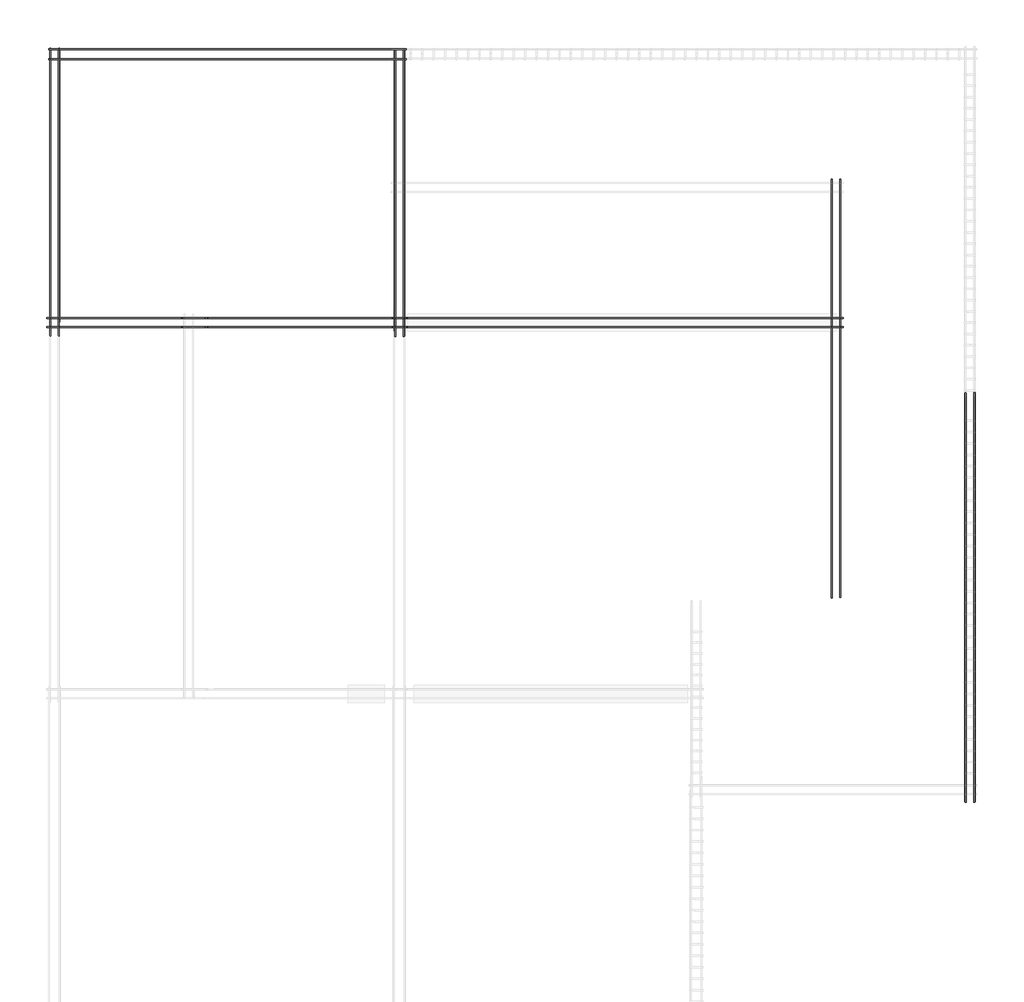
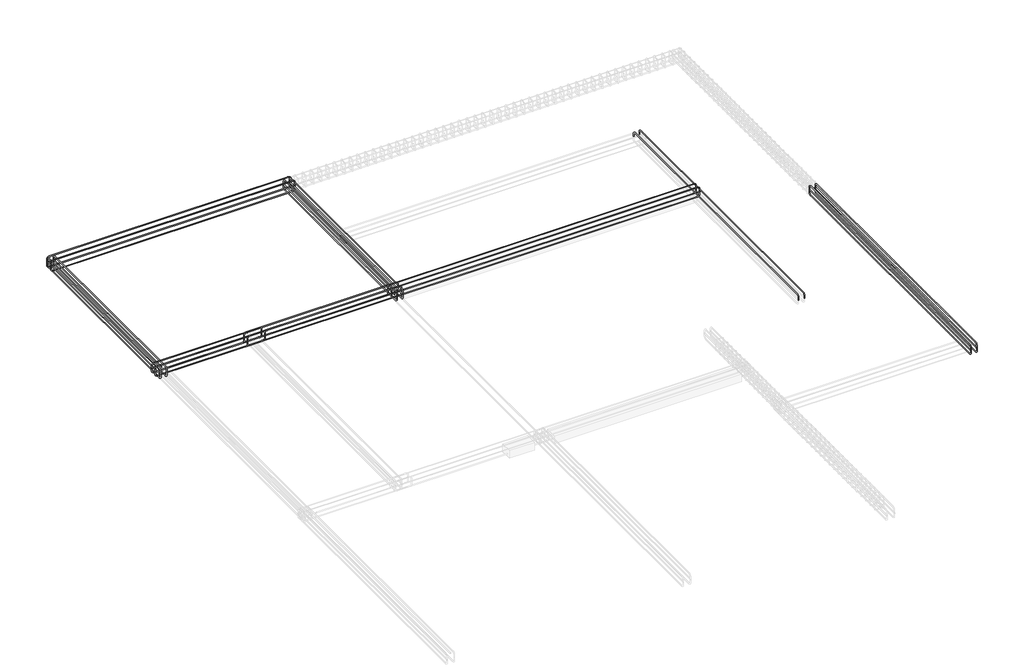
# One storey, part 4 of 5: 44 reinforcing bars.
"""IFC4 building model written with IfcOpenShell, lengths in millimetres."""

from ifc_helpers import new_model, si_unit, point, frame, origin, place, context, project, spatial, polyline, circle_curve, trimmed, segment, composite_curve, element, save
from ifc_brep_helpers import swept_disk

model = new_model("IFC4")

# Units and contexts
model_context = context("Model", 3, world=origin())
ifc_project = project(units=[si_unit("LENGTHUNIT", "METRE", prefix="MILLI")], contexts=[model_context])

# Site, building, storey
site = spatial("IfcSite", under=ifc_project)
building = spatial("IfcBuilding", under=site)
storey = spatial("IfcBuildingStorey", under=building, Elevation=0.0)

# Reinforcing bars
placement = place(None, origin())
element("IfcReinforcingBar", 1, at=placement, inside=storey, context=model_context, shape_type="SolidModel", body=[
    swept_disk(composite_curve([segment(polyline([(-10115.1918223, 13372.4913561, 314.2193272), (-10115.1918223, 13372.4913561, 365.0193272)]), True, "CONTINUOUS"), segment(trimmed(circle_curve(frame((-10159.6418223, 13372.4913561, 365.0193272), z_axis=(0.0, -1.0, 0.0), x_axis=(44.45000000000073, 0.0, 0.0)), 44.45), [point((-10115.1918223, 13372.4913561, 365.0193272))], [point((-10159.6418223, 13372.4913561, 409.4693272))], True, "CARTESIAN"), True, "CONTINUOUS"), segment(polyline([(-10159.6418223, 13372.4913561, 409.4693272), (-14737.9918223, 13372.4913561, 409.4693272)]), True, "CONTINUOUS"), segment(trimmed(circle_curve(frame((-14737.9918223, 13372.4913561, 365.0193272), z_axis=(0.0, -1.0, 0.0), x_axis=(0.0, 0.0, 44.44999999999999)), 44.45), [point((-14737.9918223, 13372.4913561, 409.4693272))], [point((-14782.4418223, 13372.4913561, 365.0193272))], True, "CARTESIAN"), True, "CONTINUOUS"), segment(polyline([(-14782.4418223, 13372.4913561, 365.0193272), (-14782.4418223, 13372.4913561, 314.2193272)]), True, "CONTINUOUS")], self_intersect=False), 6.35),
])
element("IfcReinforcingBar", 2, at=placement, inside=storey, context=model_context, shape_type="SolidModel", body=[
    swept_disk(composite_curve([segment(polyline([(-10115.1918223, 13244.7305243, 314.2193272), (-10115.1918223, 13244.7305243, 365.0193272)]), True, "CONTINUOUS"), segment(trimmed(circle_curve(frame((-10159.6418223, 13244.7305243, 365.0193272), z_axis=(0.0, -1.0, 0.0), x_axis=(44.45000000000073, 0.0, 0.0)), 44.45), [point((-10115.1918223, 13244.7305243, 365.0193272))], [point((-10159.6418223, 13244.7305243, 409.4693272))], True, "CARTESIAN"), True, "CONTINUOUS"), segment(polyline([(-10159.6418223, 13244.7305243, 409.4693272), (-14737.9918223, 13244.7305243, 409.4693272)]), True, "CONTINUOUS"), segment(trimmed(circle_curve(frame((-14737.9918223, 13244.7305243, 365.0193272), z_axis=(0.0, -1.0, 0.0), x_axis=(0.0, 0.0, 44.44999999999999)), 44.45), [point((-14737.9918223, 13244.7305243, 409.4693272))], [point((-14782.4418223, 13244.7305243, 365.0193272))], True, "CARTESIAN"), True, "CONTINUOUS"), segment(polyline([(-14782.4418223, 13244.7305243, 365.0193272), (-14782.4418223, 13244.7305243, 314.2193272)]), True, "CONTINUOUS")], self_intersect=False), 6.35),
])
element("IfcReinforcingBar", 3, at=placement, inside=storey, context=model_context, shape_type="SolidModel", body=[
    swept_disk(composite_curve([segment(polyline([(-10115.1918223, 13372.4913561, 295.3806728), (-10115.1918223, 13372.4913561, 244.5806728)]), True, "CONTINUOUS"), segment(trimmed(circle_curve(frame((-10159.6418223, 13372.4913561, 244.5806728), z_axis=(0.0, 1.0, 0.0), x_axis=(44.45000000000073, 0.0, 0.0)), 44.45), [point((-10115.1918223, 13372.4913561, 244.5806728))], [point((-10159.6418223, 13372.4913561, 200.1306728))], True, "CARTESIAN"), True, "CONTINUOUS"), segment(polyline([(-10159.6418223, 13372.4913561, 200.1306728), (-14737.9918223, 13372.4913561, 200.1306728)]), True, "CONTINUOUS"), segment(trimmed(circle_curve(frame((-14737.9918223, 13372.4913561, 244.5806728), z_axis=(0.0, 1.0, 0.0), x_axis=(0.0, 0.0, -44.44999999999999)), 44.45), [point((-14737.9918223, 13372.4913561, 200.1306728))], [point((-14782.4418223, 13372.4913561, 244.5806728))], True, "CARTESIAN"), True, "CONTINUOUS"), segment(polyline([(-14782.4418223, 13372.4913561, 244.5806728), (-14782.4418223, 13372.4913561, 295.3806728)]), True, "CONTINUOUS")], self_intersect=False), 6.35),
])
element("IfcReinforcingBar", 4, at=placement, inside=storey, context=model_context, shape_type="SolidModel", body=[
    swept_disk(composite_curve([segment(polyline([(-10115.1918223, 13244.7305243, 295.3806728), (-10115.1918223, 13244.7305243, 244.5806728)]), True, "CONTINUOUS"), segment(trimmed(circle_curve(frame((-10159.6418223, 13244.7305243, 244.5806728), z_axis=(0.0, 1.0, 0.0), x_axis=(44.45000000000073, 0.0, 0.0)), 44.45), [point((-10115.1918223, 13244.7305243, 244.5806728))], [point((-10159.6418223, 13244.7305243, 200.1306728))], True, "CARTESIAN"), True, "CONTINUOUS"), segment(polyline([(-10159.6418223, 13244.7305243, 200.1306728), (-14737.9918223, 13244.7305243, 200.1306728)]), True, "CONTINUOUS"), segment(trimmed(circle_curve(frame((-14737.9918223, 13244.7305243, 244.5806728), z_axis=(0.0, 1.0, 0.0), x_axis=(0.0, 0.0, -44.44999999999999)), 44.45), [point((-14737.9918223, 13244.7305243, 200.1306728))], [point((-14782.4418223, 13244.7305243, 244.5806728))], True, "CARTESIAN"), True, "CONTINUOUS"), segment(polyline([(-14782.4418223, 13244.7305243, 244.5806728), (-14782.4418223, 13244.7305243, 295.3806728)]), True, "CONTINUOUS")], self_intersect=False), 6.35),
])
element("IfcReinforcingBar", 5, at=placement, inside=storey, context=model_context, shape_type="SolidModel", body=[
    swept_disk(composite_curve([segment(polyline([(-10108.8418223, 13244.7305243, 304.8), (-14788.7918223, 13244.7305243, 304.8)]), True, "CONTINUOUS")], self_intersect=False), 6.35),
])
element("IfcReinforcingBar", 6, at=placement, inside=storey, context=model_context, shape_type="SolidModel", body=[
    swept_disk(composite_curve([segment(polyline([(-10108.8418223, 13372.4913561, 304.8), (-14788.7918223, 13372.4913561, 304.8)]), True, "CONTINUOUS")], self_intersect=False), 6.35),
])
element("IfcReinforcingBar", 7, at=placement, inside=storey, context=model_context, shape_type="SolidModel", body=[
    swept_disk(composite_curve([segment(polyline([(-10099.8320202, 9849.2631363, 304.2552561), (-10099.8320202, 9849.2631363, 355.0552561)]), True, "CONTINUOUS"), segment(trimmed(circle_curve(frame((-10144.2820202, 9849.2631363, 355.0552561), z_axis=(0.0, -1.0, 0.0), x_axis=(44.45000000000073, 0.0, 0.0)), 44.45), [point((-10099.8320202, 9849.2631363, 355.0552561))], [point((-10144.2820202, 9849.2631363, 399.5052561))], True, "CARTESIAN"), True, "CONTINUOUS"), segment(polyline([(-10144.2820202, 9849.2631363, 399.5052561), (-13001.0910339, 9849.2631363, 399.5052561)]), True, "CONTINUOUS"), segment(trimmed(circle_curve(frame((-13001.0910339, 9849.2631363, 355.0552561), z_axis=(0.0, -1.0, 0.0), x_axis=(0.0, 0.0, 44.44999999999999)), 44.45), [point((-13001.0910339, 9849.2631363, 399.5052561))], [point((-13045.5410339, 9849.2631363, 355.0552561))], True, "CARTESIAN"), True, "CONTINUOUS"), segment(polyline([(-13045.5410339, 9849.2631363, 355.0552561), (-13045.5410339, 9849.2631363, 304.2552561)]), True, "CONTINUOUS")], self_intersect=False), 6.35),
])
element("IfcReinforcingBar", 8, at=placement, inside=storey, context=model_context, shape_type="SolidModel", body=[
    swept_disk(composite_curve([segment(polyline([(-10099.2144386, 9736.0526241, 304.2552561), (-10099.2144386, 9736.0526241, 355.0552561)]), True, "CONTINUOUS"), segment(trimmed(circle_curve(frame((-10143.6644386, 9736.0526241, 355.0552561), z_axis=(0.0, -1.0, 0.0), x_axis=(44.45000000000073, 0.0, 0.0)), 44.45), [point((-10099.2144386, 9736.0526241, 355.0552561))], [point((-10143.6644386, 9736.0526241, 399.5052561))], True, "CARTESIAN"), True, "CONTINUOUS"), segment(polyline([(-10143.6644386, 9736.0526241, 399.5052561), (-13000.994754, 9736.0526241, 399.5052561)]), True, "CONTINUOUS"), segment(trimmed(circle_curve(frame((-13000.994754, 9736.0526241, 355.0552561), z_axis=(0.0, -1.0, 0.0), x_axis=(0.0, 0.0, 44.44999999999999)), 44.45), [point((-13000.994754, 9736.0526241, 399.5052561))], [point((-13045.444754, 9736.0526241, 355.0552561))], True, "CARTESIAN"), True, "CONTINUOUS"), segment(polyline([(-13045.444754, 9736.0526241, 355.0552561), (-13045.444754, 9736.0526241, 304.2552561)]), True, "CONTINUOUS")], self_intersect=False), 6.35),
])
element("IfcReinforcingBar", 9, at=placement, inside=storey, context=model_context, shape_type="SolidModel", body=[
    swept_disk(composite_curve([segment(polyline([(-10099.6362316, 9849.2631363, 305.3447439), (-10099.6362316, 9849.2631363, 254.5447439)]), True, "CONTINUOUS"), segment(trimmed(circle_curve(frame((-10144.0862316, 9849.2631363, 254.5447439), z_axis=(0.0, 1.0, 0.0), x_axis=(44.45000000000073, 0.0, 0.0)), 44.45), [point((-10099.6362316, 9849.2631363, 254.5447439))], [point((-10144.0862316, 9849.2631363, 210.0947439))], True, "CARTESIAN"), True, "CONTINUOUS"), segment(polyline([(-10144.0862316, 9849.2631363, 210.0947439), (-13000.8390327, 9849.2631363, 210.0947439)]), True, "CONTINUOUS"), segment(trimmed(circle_curve(frame((-13000.8390327, 9849.2631363, 254.5447439), z_axis=(0.0, 1.0, 0.0), x_axis=(0.0, 0.0, -44.44999999999999)), 44.45), [point((-13000.8390327, 9849.2631363, 210.0947439))], [point((-13045.2890327, 9849.2631363, 254.5447439))], True, "CARTESIAN"), True, "CONTINUOUS"), segment(polyline([(-13045.2890327, 9849.2631363, 254.5447439), (-13045.2890327, 9849.2631363, 305.3447439)]), True, "CONTINUOUS")], self_intersect=False), 6.35),
])
element("IfcReinforcingBar", 10, at=placement, inside=storey, context=model_context, shape_type="SolidModel", body=[
    swept_disk(composite_curve([segment(polyline([(-10098.2917322, 9736.0526241, 305.3447439), (-10098.2917322, 9736.0526241, 254.5447439)]), True, "CONTINUOUS"), segment(trimmed(circle_curve(frame((-10142.7417322, 9736.0526241, 254.5447439), z_axis=(0.0, 1.0, 0.0), x_axis=(44.45000000000073, 0.0, 0.0)), 44.45), [point((-10098.2917322, 9736.0526241, 254.5447439))], [point((-10142.7417322, 9736.0526241, 210.0947439))], True, "CARTESIAN"), True, "CONTINUOUS"), segment(polyline([(-10142.7417322, 9736.0526241, 210.0947439), (-13000.4708006, 9736.0526241, 210.0947439)]), True, "CONTINUOUS"), segment(trimmed(circle_curve(frame((-13000.4708006, 9736.0526241, 254.5447439), z_axis=(0.0, 1.0, 0.0), x_axis=(0.0, 0.0, -44.44999999999999)), 44.45), [point((-13000.4708006, 9736.0526241, 210.0947439))], [point((-13044.9208006, 9736.0526241, 254.5447439))], True, "CARTESIAN"), True, "CONTINUOUS"), segment(polyline([(-13044.9208006, 9736.0526241, 254.5447439), (-13044.9208006, 9736.0526241, 305.3447439)]), True, "CONTINUOUS")], self_intersect=False), 6.35),
])
element("IfcReinforcingBar", 11, at=placement, inside=storey, context=model_context, shape_type="SolidModel", body=[
    swept_disk(composite_curve([segment(polyline([(-10092.5417314, 9852.9828802, 304.8), (-12623.4418223, 9852.9828802, 304.8)]), True, "CONTINUOUS")], self_intersect=False), 6.35),
])
element("IfcReinforcingBar", 12, at=placement, inside=storey, context=model_context, shape_type="SolidModel", body=[
    swept_disk(composite_curve([segment(polyline([(-10091.8533466, 9732.3328802, 304.8), (-13051.6902836, 9732.3328802, 304.8)]), True, "CONTINUOUS")], self_intersect=False), 6.35),
])
element("IfcReinforcingBar", 13, at=placement, inside=storey, context=model_context, shape_type="SolidModel", body=[
    swept_disk(composite_curve([segment(polyline([(-14810.5016244, 9736.0526241, 304.2552561), (-14810.5016244, 9736.0526241, 355.0552561)]), True, "CONTINUOUS"), segment(trimmed(circle_curve(frame((-14766.0516244, 9736.0526241, 355.0552561), z_axis=(0.0, 1.0, 0.0), x_axis=(-44.45000000000073, 0.0, 0.0)), 44.45), [point((-14810.5016244, 9736.0526241, 355.0552561))], [point((-14766.0516244, 9736.0526241, 399.5052561))], True, "CARTESIAN"), True, "CONTINUOUS"), segment(polyline([(-14766.0516244, 9736.0526241, 399.5052561), (-12753.7926107, 9736.0526241, 399.5052561)]), True, "CONTINUOUS"), segment(trimmed(circle_curve(frame((-12753.7926107, 9736.0526241, 355.0552561), z_axis=(0.0, 1.0, 0.0), x_axis=(0.0, 0.0, 44.44999999999999)), 44.45), [point((-12753.7926107, 9736.0526241, 399.5052561))], [point((-12709.3426107, 9736.0526241, 355.0552561))], True, "CARTESIAN"), True, "CONTINUOUS"), segment(polyline([(-12709.3426107, 9736.0526241, 355.0552561), (-12709.3426107, 9736.0526241, 304.2552561)]), True, "CONTINUOUS")], self_intersect=False), 6.35),
])
element("IfcReinforcingBar", 14, at=placement, inside=storey, context=model_context, shape_type="SolidModel", body=[
    swept_disk(composite_curve([segment(polyline([(-14811.119206, 9849.2631363, 304.2552561), (-14811.119206, 9849.2631363, 355.0552561)]), True, "CONTINUOUS"), segment(trimmed(circle_curve(frame((-14766.669206, 9849.2631363, 355.0552561), z_axis=(0.0, 1.0, 0.0), x_axis=(-44.44999999999891, 0.0, 0.0)), 44.45), [point((-14811.119206, 9849.2631363, 355.0552561))], [point((-14766.669206, 9849.2631363, 399.5052561))], True, "CARTESIAN"), True, "CONTINUOUS"), segment(polyline([(-14766.669206, 9849.2631363, 399.5052561), (-12753.8888906, 9849.2631363, 399.5052561)]), True, "CONTINUOUS"), segment(trimmed(circle_curve(frame((-12753.8888906, 9849.2631363, 355.0552561), z_axis=(0.0, 1.0, 0.0), x_axis=(0.0, 0.0, 44.44999999999999)), 44.45), [point((-12753.8888906, 9849.2631363, 399.5052561))], [point((-12709.4388906, 9849.2631363, 355.0552561))], True, "CARTESIAN"), True, "CONTINUOUS"), segment(polyline([(-12709.4388906, 9849.2631363, 355.0552561), (-12709.4388906, 9849.2631363, 304.2552561)]), True, "CONTINUOUS")], self_intersect=False), 6.35),
])
element("IfcReinforcingBar", 15, at=placement, inside=storey, context=model_context, shape_type="SolidModel", body=[
    swept_disk(composite_curve([segment(polyline([(-14810.6974131, 9736.0526241, 305.3447439), (-14810.6974131, 9736.0526241, 254.5447439)]), True, "CONTINUOUS"), segment(trimmed(circle_curve(frame((-14766.2474131, 9736.0526241, 254.5447439), z_axis=(0.0, -1.0, 0.0), x_axis=(-44.45000000000073, 0.0, 0.0)), 44.45), [point((-14810.6974131, 9736.0526241, 254.5447439))], [point((-14766.2474131, 9736.0526241, 210.0947439))], True, "CARTESIAN"), True, "CONTINUOUS"), segment(polyline([(-14766.2474131, 9736.0526241, 210.0947439), (-12754.044612, 9736.0526241, 210.0947439)]), True, "CONTINUOUS"), segment(trimmed(circle_curve(frame((-12754.044612, 9736.0526241, 254.5447439), z_axis=(0.0, -1.0, 0.0), x_axis=(0.0, 0.0, -44.44999999999999)), 44.45), [point((-12754.044612, 9736.0526241, 210.0947439))], [point((-12709.594612, 9736.0526241, 254.5447439))], True, "CARTESIAN"), True, "CONTINUOUS"), segment(polyline([(-12709.594612, 9736.0526241, 254.5447439), (-12709.594612, 9736.0526241, 305.3447439)]), True, "CONTINUOUS")], self_intersect=False), 6.35),
])
element("IfcReinforcingBar", 16, at=placement, inside=storey, context=model_context, shape_type="SolidModel", body=[
    swept_disk(composite_curve([segment(polyline([(-14812.0419124, 9849.2631363, 305.3447439), (-14812.0419124, 9849.2631363, 254.5447439)]), True, "CONTINUOUS"), segment(trimmed(circle_curve(frame((-14767.5919124, 9849.2631363, 254.5447439), z_axis=(0.0, -1.0, 0.0), x_axis=(-44.45000000000073, 0.0, 0.0)), 44.45), [point((-14812.0419124, 9849.2631363, 254.5447439))], [point((-14767.5919124, 9849.2631363, 210.0947439))], True, "CARTESIAN"), True, "CONTINUOUS"), segment(polyline([(-14767.5919124, 9849.2631363, 210.0947439), (-12754.4128441, 9849.2631363, 210.0947439)]), True, "CONTINUOUS"), segment(trimmed(circle_curve(frame((-12754.4128441, 9849.2631363, 254.5447439), z_axis=(0.0, -1.0, 0.0), x_axis=(0.0, 0.0, -44.44999999999999)), 44.45), [point((-12754.4128441, 9849.2631363, 210.0947439))], [point((-12709.9628441, 9849.2631363, 254.5447439))], True, "CARTESIAN"), True, "CONTINUOUS"), segment(polyline([(-12709.9628441, 9849.2631363, 254.5447439), (-12709.9628441, 9849.2631363, 305.3447439)]), True, "CONTINUOUS")], self_intersect=False), 6.35),
])
element("IfcReinforcingBar", 17, at=placement, inside=storey, context=model_context, shape_type="SolidModel", body=[
    swept_disk(composite_curve([segment(polyline([(-14534.7918223, 9732.3328802, 304.8), (-13131.4418223, 9732.3328802, 304.8)]), True, "CONTINUOUS")], self_intersect=False), 6.35),
])
element("IfcReinforcingBar", 18, at=placement, inside=storey, context=model_context, shape_type="SolidModel", body=[
    swept_disk(composite_curve([segment(polyline([(-14818.480298, 9852.9828802, 304.8), (-12703.1933611, 9852.9828802, 304.8)]), True, "CONTINUOUS")], self_intersect=False), 6.35),
])
element("IfcReinforcingBar", 19, at=placement, inside=storey, context=model_context, shape_type="SolidModel", body=[
    swept_disk(composite_curve([segment(polyline([(-4392.9854997, 9849.2631363, 304.2552561), (-4392.9854997, 9849.2631363, 355.0552561)]), True, "CONTINUOUS"), segment(trimmed(circle_curve(frame((-4437.4354997, 9849.2631363, 355.0552561), z_axis=(0.0, -1.0, 0.0), x_axis=(44.44999999999982, 0.0, 0.0)), 44.45), [point((-4392.9854997, 9849.2631363, 355.0552561))], [point((-4437.4354997, 9849.2631363, 399.5052561))], True, "CARTESIAN"), True, "CONTINUOUS"), segment(polyline([(-4437.4354997, 9849.2631363, 399.5052561), (-10245.1910339, 9849.2631363, 399.5052561)]), True, "CONTINUOUS"), segment(trimmed(circle_curve(frame((-10245.1910339, 9849.2631363, 355.0552561), z_axis=(0.0, -1.0, 0.0), x_axis=(0.0, 0.0, 44.44999999999999)), 44.45), [point((-10245.1910339, 9849.2631363, 399.5052561))], [point((-10289.6410339, 9849.2631363, 355.0552561))], True, "CARTESIAN"), True, "CONTINUOUS"), segment(polyline([(-10289.6410339, 9849.2631363, 355.0552561), (-10289.6410339, 9849.2631363, 304.2552561)]), True, "CONTINUOUS")], self_intersect=False), 6.35),
])
element("IfcReinforcingBar", 20, at=placement, inside=storey, context=model_context, shape_type="SolidModel", body=[
    swept_disk(composite_curve([segment(polyline([(-4393.5875013, 9736.0526241, 304.2552561), (-4393.5875013, 9736.0526241, 355.0552561)]), True, "CONTINUOUS"), segment(trimmed(circle_curve(frame((-4438.0375013, 9736.0526241, 355.0552561), z_axis=(0.0, -1.0, 0.0), x_axis=(44.44999999999982, 0.0, 0.0)), 44.45), [point((-4393.5875013, 9736.0526241, 355.0552561))], [point((-4438.0375013, 9736.0526241, 399.5052561))], True, "CARTESIAN"), True, "CONTINUOUS"), segment(polyline([(-4438.0375013, 9736.0526241, 399.5052561), (-10245.094754, 9736.0526241, 399.5052561)]), True, "CONTINUOUS"), segment(trimmed(circle_curve(frame((-10245.094754, 9736.0526241, 355.0552561), z_axis=(0.0, -1.0, 0.0), x_axis=(0.0, 0.0, 44.44999999999999)), 44.45), [point((-10245.094754, 9736.0526241, 399.5052561))], [point((-10289.544754, 9736.0526241, 355.0552561))], True, "CARTESIAN"), True, "CONTINUOUS"), segment(polyline([(-10289.544754, 9736.0526241, 355.0552561), (-10289.544754, 9736.0526241, 304.2552561)]), True, "CONTINUOUS")], self_intersect=False), 6.35),
])
element("IfcReinforcingBar", 21, at=placement, inside=storey, context=model_context, shape_type="SolidModel", body=[
    swept_disk(composite_curve([segment(polyline([(-4394.1639641, 9849.2631363, 305.3447439), (-4394.1639641, 9849.2631363, 254.5447439)]), True, "CONTINUOUS"), segment(trimmed(circle_curve(frame((-4438.6139641, 9849.2631363, 254.5447439), z_axis=(0.0, 1.0, 0.0), x_axis=(44.44999999999982, 0.0, 0.0)), 44.45), [point((-4394.1639641, 9849.2631363, 254.5447439))], [point((-4438.6139641, 9849.2631363, 210.0947439))], True, "CARTESIAN"), True, "CONTINUOUS"), segment(polyline([(-4438.6139641, 9849.2631363, 210.0947439), (-10244.9390327, 9849.2631363, 210.0947439)]), True, "CONTINUOUS"), segment(trimmed(circle_curve(frame((-10244.9390327, 9849.2631363, 254.5447439), z_axis=(0.0, 1.0, 0.0), x_axis=(0.0, 0.0, -44.44999999999999)), 44.45), [point((-10244.9390327, 9849.2631363, 210.0947439))], [point((-10289.3890327, 9849.2631363, 254.5447439))], True, "CARTESIAN"), True, "CONTINUOUS"), segment(polyline([(-10289.3890327, 9849.2631363, 254.5447439), (-10289.3890327, 9849.2631363, 305.3447439)]), True, "CONTINUOUS")], self_intersect=False), 6.35),
])
element("IfcReinforcingBar", 22, at=placement, inside=storey, context=model_context, shape_type="SolidModel", body=[
    swept_disk(composite_curve([segment(polyline([(-4394.4425489, 9736.0526241, 305.3447439), (-4394.4425489, 9736.0526241, 254.5447439)]), True, "CONTINUOUS"), segment(trimmed(circle_curve(frame((-4438.8925489, 9736.0526241, 254.5447439), z_axis=(0.0, 1.0, 0.0), x_axis=(44.45000000000073, 0.0, 0.0)), 44.45), [point((-4394.4425489, 9736.0526241, 254.5447439))], [point((-4438.8925489, 9736.0526241, 210.0947439))], True, "CARTESIAN"), True, "CONTINUOUS"), segment(polyline([(-4438.8925489, 9736.0526241, 210.0947439), (-10244.5708006, 9736.0526241, 210.0947439)]), True, "CONTINUOUS"), segment(trimmed(circle_curve(frame((-10244.5708006, 9736.0526241, 254.5447439), z_axis=(0.0, 1.0, 0.0), x_axis=(0.0, 0.0, -44.44999999999999)), 44.45), [point((-10244.5708006, 9736.0526241, 210.0947439))], [point((-10289.0208006, 9736.0526241, 254.5447439))], True, "CARTESIAN"), True, "CONTINUOUS"), segment(polyline([(-10289.0208006, 9736.0526241, 254.5447439), (-10289.0208006, 9736.0526241, 305.3447439)]), True, "CONTINUOUS")], self_intersect=False), 6.35),
])
element("IfcReinforcingBar", 23, at=placement, inside=storey, context=model_context, shape_type="SolidModel", body=[
    swept_disk(composite_curve([segment(polyline([(-4387.2848989, 9852.9828802, 304.8), (-10295.4820168, 9852.9828802, 304.8)]), True, "CONTINUOUS")], self_intersect=False), 6.35),
])
element("IfcReinforcingBar", 24, at=placement, inside=storey, context=model_context, shape_type="SolidModel", body=[
    swept_disk(composite_curve([segment(polyline([(-4387.1707513, 9732.3328802, 304.8), (-10295.7902836, 9732.3328802, 304.8)]), True, "CONTINUOUS")], self_intersect=False), 6.35),
])
element("IfcReinforcingBar", 25, at=placement, inside=storey, context=model_context, shape_type="SolidModel", body=[
    swept_disk(composite_curve([segment(polyline([(-10254.3470784, 13369.123342, 304.2552561), (-10254.3470784, 13369.123342, 355.0552561)]), True, "CONTINUOUS"), segment(trimmed(circle_curve(frame((-10254.3470784, 13324.673342, 355.0552561), z_axis=(1.0, 0.0, 0.0), x_axis=(0.0, 44.45000000000073, 0.0)), 44.45), [point((-10254.3470784, 13369.123342, 355.0552561))], [point((-10254.3470784, 13324.673342, 399.5052561))], True, "CARTESIAN"), True, "CONTINUOUS"), segment(polyline([(-10254.3470784, 13324.673342, 399.5052561), (-10254.3470784, 9660.4683576, 399.5052561)]), True, "CONTINUOUS"), segment(trimmed(circle_curve(frame((-10254.3470784, 9660.4683576, 355.0552561), z_axis=(1.0, 0.0, 0.0), x_axis=(0.0, 0.0, 44.44999999999999)), 44.45), [point((-10254.3470784, 9660.4683576, 399.5052561))], [point((-10254.3470784, 9616.0183576, 355.0552561))], True, "CARTESIAN"), True, "CONTINUOUS"), segment(polyline([(-10254.3470784, 9616.0183576, 355.0552561), (-10254.3470784, 9616.0183576, 304.2552561)]), True, "CONTINUOUS")], self_intersect=False), 6.35),
])
element("IfcReinforcingBar", 26, at=placement, inside=storey, context=model_context, shape_type="SolidModel", body=[
    swept_disk(composite_curve([segment(polyline([(-10141.1365662, 13368.9893399, 304.2552561), (-10141.1365662, 13368.9893399, 355.0552561)]), True, "CONTINUOUS"), segment(trimmed(circle_curve(frame((-10141.1365662, 13324.5393399, 355.0552561), z_axis=(1.0, 0.0, 0.0), x_axis=(0.0, 44.44999999999891, 0.0)), 44.45), [point((-10141.1365662, 13368.9893399, 355.0552561))], [point((-10141.1365662, 13324.5393399, 399.5052561))], True, "CARTESIAN"), True, "CONTINUOUS"), segment(polyline([(-10141.1365662, 13324.5393399, 399.5052561), (-10141.1365662, 9660.4683576, 399.5052561)]), True, "CONTINUOUS"), segment(trimmed(circle_curve(frame((-10141.1365662, 9660.4683576, 355.0552561), z_axis=(1.0, 0.0, 0.0), x_axis=(0.0, 0.0, 44.44999999999999)), 44.45), [point((-10141.1365662, 9660.4683576, 399.5052561))], [point((-10141.1365662, 9616.0183576, 355.0552561))], True, "CARTESIAN"), True, "CONTINUOUS"), segment(polyline([(-10141.1365662, 9616.0183576, 355.0552561), (-10141.1365662, 9616.0183576, 304.2552561)]), True, "CONTINUOUS")], self_intersect=False), 6.35),
])
element("IfcReinforcingBar", 27, at=placement, inside=storey, context=model_context, shape_type="SolidModel", body=[
    swept_disk(composite_curve([segment(polyline([(-10254.3470784, 13368.3917697, 305.3447439), (-10254.3470784, 13368.3917697, 254.5447439)]), True, "CONTINUOUS"), segment(trimmed(circle_curve(frame((-10254.3470784, 13323.9417697, 254.5447439), z_axis=(-1.0, 0.0, 0.0), x_axis=(0.0, 44.44999999999891, 0.0)), 44.45), [point((-10254.3470784, 13368.3917697, 254.5447439))], [point((-10254.3470784, 13323.9417697, 210.0947439))], True, "CARTESIAN"), True, "CONTINUOUS"), segment(polyline([(-10254.3470784, 13323.9417697, 210.0947439), (-10254.3470784, 9658.9413566, 210.0947439)]), True, "CONTINUOUS"), segment(trimmed(circle_curve(frame((-10254.3470784, 9658.9413566, 254.5447439), z_axis=(-1.0, 0.0, 0.0), x_axis=(0.0, 0.0, -44.44999999999999)), 44.45), [point((-10254.3470784, 9658.9413566, 210.0947439))], [point((-10254.3470784, 9614.4913566, 254.5447439))], True, "CARTESIAN"), True, "CONTINUOUS"), segment(polyline([(-10254.3470784, 9614.4913566, 254.5447439), (-10254.3470784, 9614.4913566, 305.3447439)]), True, "CONTINUOUS")], self_intersect=False), 6.35),
])
element("IfcReinforcingBar", 28, at=placement, inside=storey, context=model_context, shape_type="SolidModel", body=[
    swept_disk(composite_curve([segment(polyline([(-10141.1365662, 13368.1534656, 305.3447439), (-10141.1365662, 13368.1534656, 254.5447439)]), True, "CONTINUOUS"), segment(trimmed(circle_curve(frame((-10141.1365662, 13323.7034656, 254.5447439), z_axis=(-1.0, 0.0, 0.0), x_axis=(0.0, 44.45000000000073, 0.0)), 44.45), [point((-10141.1365662, 13368.1534656, 254.5447439))], [point((-10141.1365662, 13323.7034656, 210.0947439))], True, "CARTESIAN"), True, "CONTINUOUS"), segment(polyline([(-10141.1365662, 13323.7034656, 210.0947439), (-10141.1365662, 9659.4503569, 210.0947439)]), True, "CONTINUOUS"), segment(trimmed(circle_curve(frame((-10141.1365662, 9659.4503569, 254.5447439), z_axis=(-1.0, 0.0, 0.0), x_axis=(0.0, 0.0, -44.44999999999999)), 44.45), [point((-10141.1365662, 9659.4503569, 210.0947439))], [point((-10141.1365662, 9615.0003569, 254.5447439))], True, "CARTESIAN"), True, "CONTINUOUS"), segment(polyline([(-10141.1365662, 9615.0003569, 254.5447439), (-10141.1365662, 9615.0003569, 305.3447439)]), True, "CONTINUOUS")], self_intersect=False), 6.35),
])
element("IfcReinforcingBar", 29, at=placement, inside=storey, context=model_context, shape_type="SolidModel", body=[
    swept_disk(composite_curve([segment(polyline([(-10258.0668223, 13375.0932689, 304.8), (-10258.0668223, 9684.1321282, 304.8)]), True, "CONTINUOUS")], self_intersect=False), 6.35),
])
element("IfcReinforcingBar", 30, at=placement, inside=storey, context=model_context, shape_type="SolidModel", body=[
    swept_disk(composite_curve([segment(polyline([(-10137.4168223, 13374.9581807, 304.8), (-10137.4168223, 9618.4094189, 304.8)]), True, "CONTINUOUS")], self_intersect=False), 6.35),
])
element("IfcReinforcingBar", 31, at=placement, inside=storey, context=model_context, shape_type="SolidModel", body=[
    swept_disk(composite_curve([segment(polyline([(-14769.1970784, 13380.4078802, 304.2552561), (-14769.1970784, 13380.4078802, 355.0552561)]), True, "CONTINUOUS"), segment(trimmed(circle_curve(frame((-14769.1970784, 13335.9578802, 355.0552561), z_axis=(1.0, 0.0, 0.0), x_axis=(0.0, 44.45000000000073, 0.0)), 44.45), [point((-14769.1970784, 13380.4078802, 355.0552561))], [point((-14769.1970784, 13335.9578802, 399.5052561))], True, "CARTESIAN"), True, "CONTINUOUS"), segment(polyline([(-14769.1970784, 13335.9578802, 399.5052561), (-14769.1970784, 9669.0086686, 399.5052561)]), True, "CONTINUOUS"), segment(trimmed(circle_curve(frame((-14769.1970784, 9669.0086686, 355.0552561), z_axis=(1.0, 0.0, 0.0), x_axis=(0.0, 0.0, 44.44999999999999)), 44.45), [point((-14769.1970784, 9669.0086686, 399.5052561))], [point((-14769.1970784, 9624.5586686, 355.0552561))], True, "CARTESIAN"), True, "CONTINUOUS"), segment(polyline([(-14769.1970784, 9624.5586686, 355.0552561), (-14769.1970784, 9624.5586686, 304.2552561)]), True, "CONTINUOUS")], self_intersect=False), 6.35),
])
element("IfcReinforcingBar", 32, at=placement, inside=storey, context=model_context, shape_type="SolidModel", body=[
    swept_disk(composite_curve([segment(polyline([(-14655.9865662, 13380.4078802, 304.2552561), (-14655.9865662, 13380.4078802, 355.0552561)]), True, "CONTINUOUS"), segment(trimmed(circle_curve(frame((-14655.9865662, 13335.9578802, 355.0552561), z_axis=(1.0, 0.0, 0.0), x_axis=(0.0, 44.45000000000073, 0.0)), 44.45), [point((-14655.9865662, 13380.4078802, 355.0552561))], [point((-14655.9865662, 13335.9578802, 399.5052561))], True, "CARTESIAN"), True, "CONTINUOUS"), segment(polyline([(-14655.9865662, 13335.9578802, 399.5052561), (-14655.9865662, 9669.1049485, 399.5052561)]), True, "CONTINUOUS"), segment(trimmed(circle_curve(frame((-14655.9865662, 9669.1049485, 355.0552561), z_axis=(1.0, 0.0, 0.0), x_axis=(0.0, 0.0, 44.44999999999999)), 44.45), [point((-14655.9865662, 9669.1049485, 399.5052561))], [point((-14655.9865662, 9624.6549485, 355.0552561))], True, "CARTESIAN"), True, "CONTINUOUS"), segment(polyline([(-14655.9865662, 9624.6549485, 355.0552561), (-14655.9865662, 9624.6549485, 304.2552561)]), True, "CONTINUOUS")], self_intersect=False), 6.35),
])
element("IfcReinforcingBar", 33, at=placement, inside=storey, context=model_context, shape_type="SolidModel", body=[
    swept_disk(composite_curve([segment(polyline([(-14769.1970784, 13380.4078802, 305.3447439), (-14769.1970784, 13380.4078802, 254.5447439)]), True, "CONTINUOUS"), segment(trimmed(circle_curve(frame((-14769.1970784, 13335.9578802, 254.5447439), z_axis=(-1.0, 0.0, 0.0), x_axis=(0.0, 44.45000000000073, 0.0)), 44.45), [point((-14769.1970784, 13380.4078802, 254.5447439))], [point((-14769.1970784, 13335.9578802, 210.0947439))], True, "CARTESIAN"), True, "CONTINUOUS"), segment(polyline([(-14769.1970784, 13335.9578802, 210.0947439), (-14769.1970784, 9669.2606698, 210.0947439)]), True, "CONTINUOUS"), segment(trimmed(circle_curve(frame((-14769.1970784, 9669.2606698, 254.5447439), z_axis=(-1.0, 0.0, 0.0), x_axis=(0.0, 0.0, -44.44999999999999)), 44.45), [point((-14769.1970784, 9669.2606698, 210.0947439))], [point((-14769.1970784, 9624.8106698, 254.5447439))], True, "CARTESIAN"), True, "CONTINUOUS"), segment(polyline([(-14769.1970784, 9624.8106698, 254.5447439), (-14769.1970784, 9624.8106698, 305.3447439)]), True, "CONTINUOUS")], self_intersect=False), 6.35),
])
element("IfcReinforcingBar", 34, at=placement, inside=storey, context=model_context, shape_type="SolidModel", body=[
    swept_disk(composite_curve([segment(polyline([(-14655.9865662, 13380.4078802, 305.3447439), (-14655.9865662, 13380.4078802, 254.5447439)]), True, "CONTINUOUS"), segment(trimmed(circle_curve(frame((-14655.9865662, 13335.9578802, 254.5447439), z_axis=(-1.0, 0.0, 0.0), x_axis=(0.0, 44.45000000000073, 0.0)), 44.45), [point((-14655.9865662, 13380.4078802, 254.5447439))], [point((-14655.9865662, 13335.9578802, 210.0947439))], True, "CARTESIAN"), True, "CONTINUOUS"), segment(polyline([(-14655.9865662, 13335.9578802, 210.0947439), (-14655.9865662, 9669.6289019, 210.0947439)]), True, "CONTINUOUS"), segment(trimmed(circle_curve(frame((-14655.9865662, 9669.6289019, 254.5447439), z_axis=(-1.0, 0.0, 0.0), x_axis=(0.0, 0.0, -44.44999999999999)), 44.45), [point((-14655.9865662, 9669.6289019, 210.0947439))], [point((-14655.9865662, 9625.1789019, 254.5447439))], True, "CARTESIAN"), True, "CONTINUOUS"), segment(polyline([(-14655.9865662, 9625.1789019, 254.5447439), (-14655.9865662, 9625.1789019, 305.3447439)]), True, "CONTINUOUS")], self_intersect=False), 6.35),
])
element("IfcReinforcingBar", 35, at=placement, inside=storey, context=model_context, shape_type="SolidModel", body=[
    swept_disk(composite_curve([segment(polyline([(-14772.9168223, 13386.7578802, 304.8), (-14772.9168223, 9657.8864045, 304.8)]), True, "CONTINUOUS")], self_intersect=False), 6.35),
])
element("IfcReinforcingBar", 36, at=placement, inside=storey, context=model_context, shape_type="SolidModel", body=[
    swept_disk(composite_curve([segment(polyline([(-14652.2668223, 13386.7578802, 304.8), (-14652.2668223, 9799.1626239, 304.8)]), True, "CONTINUOUS")], self_intersect=False), 6.35),
])
element("IfcReinforcingBar", 37, at=placement, inside=storey, context=model_context, shape_type="SolidModel", body=[
    swept_disk(composite_curve([segment(polyline([(-4426.1365662, 6196.2083855, 304.2552561), (-4426.1365662, 6196.2083855, 355.0552561)]), True, "CONTINUOUS"), segment(trimmed(circle_curve(frame((-4426.1365662, 6240.6583855, 355.0552561), z_axis=(-1.0, 0.0, 0.0), x_axis=(0.0, -44.44999999999982, 0.0)), 44.45), [point((-4426.1365662, 6196.2083855, 355.0552561))], [point((-4426.1365662, 6240.6583855, 399.5052561))], True, "CARTESIAN"), True, "CONTINUOUS"), segment(polyline([(-4426.1365662, 6240.6583855, 399.5052561), (-4426.1365662, 11620.8030086, 399.5052561)]), True, "CONTINUOUS"), segment(trimmed(circle_curve(frame((-4426.1365662, 11620.8030086, 355.0552561), z_axis=(-1.0, 0.0, 0.0), x_axis=(0.0, 0.0, 44.44999999999999)), 44.45), [point((-4426.1365662, 11620.8030086, 399.5052561))], [point((-4426.1365662, 11665.2530086, 355.0552561))], True, "CARTESIAN"), True, "CONTINUOUS"), segment(polyline([(-4426.1365662, 11665.2530086, 355.0552561), (-4426.1365662, 11665.2530086, 304.2552561)]), True, "CONTINUOUS")], self_intersect=False), 6.35),
])
element("IfcReinforcingBar", 38, at=placement, inside=storey, context=model_context, shape_type="SolidModel", body=[
    swept_disk(composite_curve([segment(polyline([(-4539.3470784, 6194.4923333, 304.2552561), (-4539.3470784, 6194.4923333, 355.0552561)]), True, "CONTINUOUS"), segment(trimmed(circle_curve(frame((-4539.3470784, 6238.9423333, 355.0552561), z_axis=(-1.0, 0.0, 0.0), x_axis=(0.0, -44.45000000000073, 0.0)), 44.45), [point((-4539.3470784, 6194.4923333, 355.0552561))], [point((-4539.3470784, 6238.9423333, 399.5052561))], True, "CARTESIAN"), True, "CONTINUOUS"), segment(polyline([(-4539.3470784, 6238.9423333, 399.5052561), (-4539.3470784, 11620.7067287, 399.5052561)]), True, "CONTINUOUS"), segment(trimmed(circle_curve(frame((-4539.3470784, 11620.7067287, 355.0552561), z_axis=(-1.0, 0.0, 0.0), x_axis=(0.0, 0.0, 44.44999999999999)), 44.45), [point((-4539.3470784, 11620.7067287, 399.5052561))], [point((-4539.3470784, 11665.1567287, 355.0552561))], True, "CARTESIAN"), True, "CONTINUOUS"), segment(polyline([(-4539.3470784, 11665.1567287, 355.0552561), (-4539.3470784, 11665.1567287, 304.2552561)]), True, "CONTINUOUS")], self_intersect=False), 6.35),
])
element("IfcReinforcingBar", 39, at=placement, inside=storey, context=model_context, shape_type="SolidModel", body=[
    swept_disk(composite_curve([segment(polyline([(-2673.5365662, 3516.5083855, 304.2552561), (-2673.5365662, 3516.5083855, 355.0552561)]), True, "CONTINUOUS"), segment(trimmed(circle_curve(frame((-2673.5365662, 3560.9583855, 355.0552561), z_axis=(-1.0, 0.0, 0.0), x_axis=(0.0, -44.45000000000027, 0.0)), 44.45), [point((-2673.5365662, 3516.5083855, 355.0552561))], [point((-2673.5365662, 3560.9583855, 399.5052561))], True, "CARTESIAN"), True, "CONTINUOUS"), segment(polyline([(-2673.5365662, 3560.9583855, 399.5052561), (-2673.5365662, 8824.1070918, 399.5052561)]), True, "CONTINUOUS"), segment(trimmed(circle_curve(frame((-2673.5365662, 8824.1070918, 355.0552561), z_axis=(-1.0, 0.0, 0.0), x_axis=(0.0, 0.0, 44.44999999999999)), 44.45), [point((-2673.5365662, 8824.1070918, 399.5052561))], [point((-2673.5365662, 8868.5570918, 355.0552561))], True, "CARTESIAN"), True, "CONTINUOUS"), segment(polyline([(-2673.5365662, 8868.5570918, 355.0552561), (-2673.5365662, 8868.5570918, 304.2552561)]), True, "CONTINUOUS")], self_intersect=False), 6.35),
])
element("IfcReinforcingBar", 40, at=placement, inside=storey, context=model_context, shape_type="SolidModel", body=[
    swept_disk(composite_curve([segment(polyline([(-2786.7470784, 3514.7923333, 304.2552561), (-2786.7470784, 3514.7923333, 355.0552561)]), True, "CONTINUOUS"), segment(trimmed(circle_curve(frame((-2786.7470784, 3559.2423333, 355.0552561), z_axis=(-1.0, 0.0, 0.0), x_axis=(0.0, -44.45000000000027, 0.0)), 44.45), [point((-2786.7470784, 3514.7923333, 355.0552561))], [point((-2786.7470784, 3559.2423333, 399.5052561))], True, "CARTESIAN"), True, "CONTINUOUS"), segment(polyline([(-2786.7470784, 3559.2423333, 399.5052561), (-2786.7470784, 8824.0108119, 399.5052561)]), True, "CONTINUOUS"), segment(trimmed(circle_curve(frame((-2786.7470784, 8824.0108119, 355.0552561), z_axis=(-1.0, 0.0, 0.0), x_axis=(0.0, 0.0, 44.44999999999999)), 44.45), [point((-2786.7470784, 8824.0108119, 399.5052561))], [point((-2786.7470784, 8868.4608119, 355.0552561))], True, "CARTESIAN"), True, "CONTINUOUS"), segment(polyline([(-2786.7470784, 8868.4608119, 355.0552561), (-2786.7470784, 8868.4608119, 304.2552561)]), True, "CONTINUOUS")], self_intersect=False), 6.35),
])
element("IfcReinforcingBar", 41, at=placement, inside=storey, context=model_context, shape_type="SolidModel", body=[
    swept_disk(composite_curve([segment(polyline([(-2673.5365662, 3513.4570312, 305.3447439), (-2673.5365662, 3513.4570312, 254.5447439)]), True, "CONTINUOUS"), segment(trimmed(circle_curve(frame((-2673.5365662, 3557.9070312, 254.5447439), z_axis=(1.0, 0.0, 0.0), x_axis=(0.0, -44.44999999999982, 0.0)), 44.45), [point((-2673.5365662, 3513.4570312, 254.5447439))], [point((-2673.5365662, 3557.9070312, 210.0947439))], True, "CARTESIAN"), True, "CONTINUOUS"), segment(polyline([(-2673.5365662, 3557.9070312, 210.0947439), (-2673.5365662, 8823.8550905, 210.0947439)]), True, "CONTINUOUS"), segment(trimmed(circle_curve(frame((-2673.5365662, 8823.8550905, 254.5447439), z_axis=(1.0, 0.0, 0.0), x_axis=(0.0, 0.0, -44.44999999999999)), 44.45), [point((-2673.5365662, 8823.8550905, 210.0947439))], [point((-2673.5365662, 8868.3050905, 254.5447439))], True, "CARTESIAN"), True, "CONTINUOUS"), segment(polyline([(-2673.5365662, 8868.3050905, 254.5447439), (-2673.5365662, 8868.3050905, 305.3447439)]), True, "CONTINUOUS")], self_intersect=False), 6.35),
])
element("IfcReinforcingBar", 42, at=placement, inside=storey, context=model_context, shape_type="SolidModel", body=[
    swept_disk(composite_curve([segment(polyline([(-2786.7470784, 3515.8320827, 305.3447439), (-2786.7470784, 3515.8320827, 254.5447439)]), True, "CONTINUOUS"), segment(trimmed(circle_curve(frame((-2786.7470784, 3560.2820827, 254.5447439), z_axis=(1.0, 0.0, 0.0), x_axis=(0.0, -44.45000000000027, 0.0)), 44.45), [point((-2786.7470784, 3515.8320827, 254.5447439))], [point((-2786.7470784, 3560.2820827, 210.0947439))], True, "CARTESIAN"), True, "CONTINUOUS"), segment(polyline([(-2786.7470784, 3560.2820827, 210.0947439), (-2786.7470784, 8823.4868584, 210.0947439)]), True, "CONTINUOUS"), segment(trimmed(circle_curve(frame((-2786.7470784, 8823.4868584, 254.5447439), z_axis=(1.0, 0.0, 0.0), x_axis=(0.0, 0.0, -44.44999999999999)), 44.45), [point((-2786.7470784, 8823.4868584, 210.0947439))], [point((-2786.7470784, 8867.9368584, 254.5447439))], True, "CARTESIAN"), True, "CONTINUOUS"), segment(polyline([(-2786.7470784, 8867.9368584, 254.5447439), (-2786.7470784, 8867.9368584, 305.3447439)]), True, "CONTINUOUS")], self_intersect=False), 6.35),
])
element("IfcReinforcingBar", 43, at=placement, inside=storey, context=model_context, shape_type="SolidModel", body=[
    swept_disk(composite_curve([segment(polyline([(-2669.8168223, 3518.8578802, 304.8), (-2669.8168223, 8879.1074706, 304.8)]), True, "CONTINUOUS")], self_intersect=False), 6.35),
])
element("IfcReinforcingBar", 44, at=placement, inside=storey, context=model_context, shape_type="SolidModel", body=[
    swept_disk(composite_curve([segment(polyline([(-2790.4668223, 3518.8578802, 304.8), (-2790.4668223, 8867.2133353, 304.8)]), True, "CONTINUOUS")], self_intersect=False), 6.35),
])

save(model, "model.ifc")

# Revit data of these elements
# Elements 1, 2, 3, 4, 5, 6, 7, 8, 9, 10, 11, 12, 13, 14, 15, 16, 17, 18, 19, 20, 21, 22, 23, 24, 25, 26, 27, 28, 29, 30, 31, 32, 33, 34, 35, 36, 37, 38, 39, 40, 41, 42, 43, 44 (IfcReinforcingBar)
#   Phase Created = New Construction
